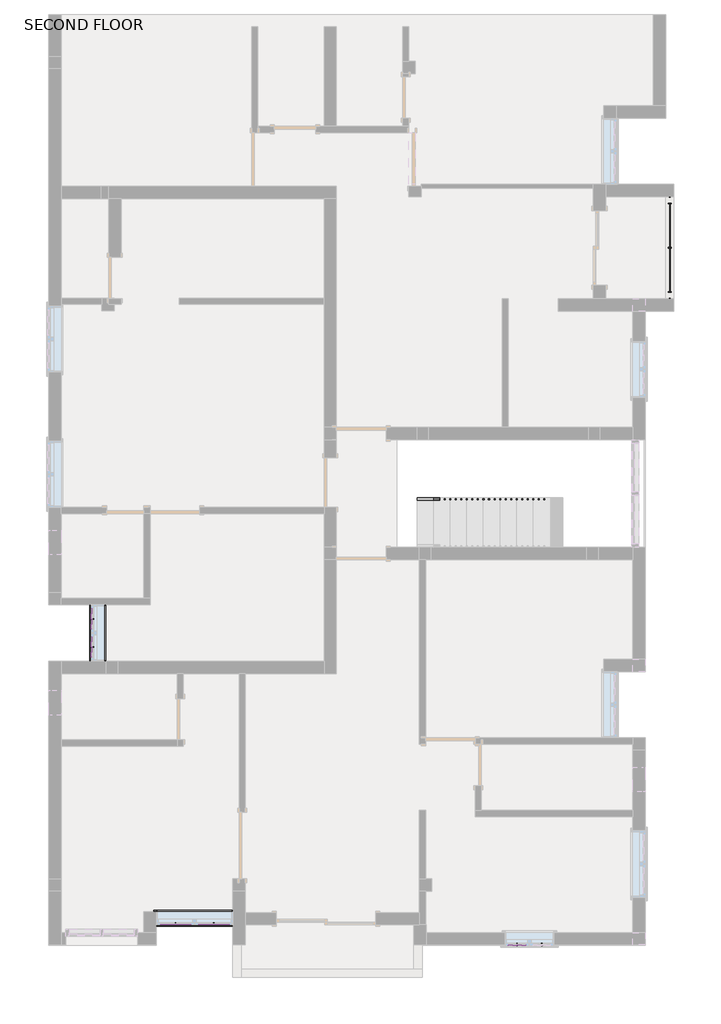
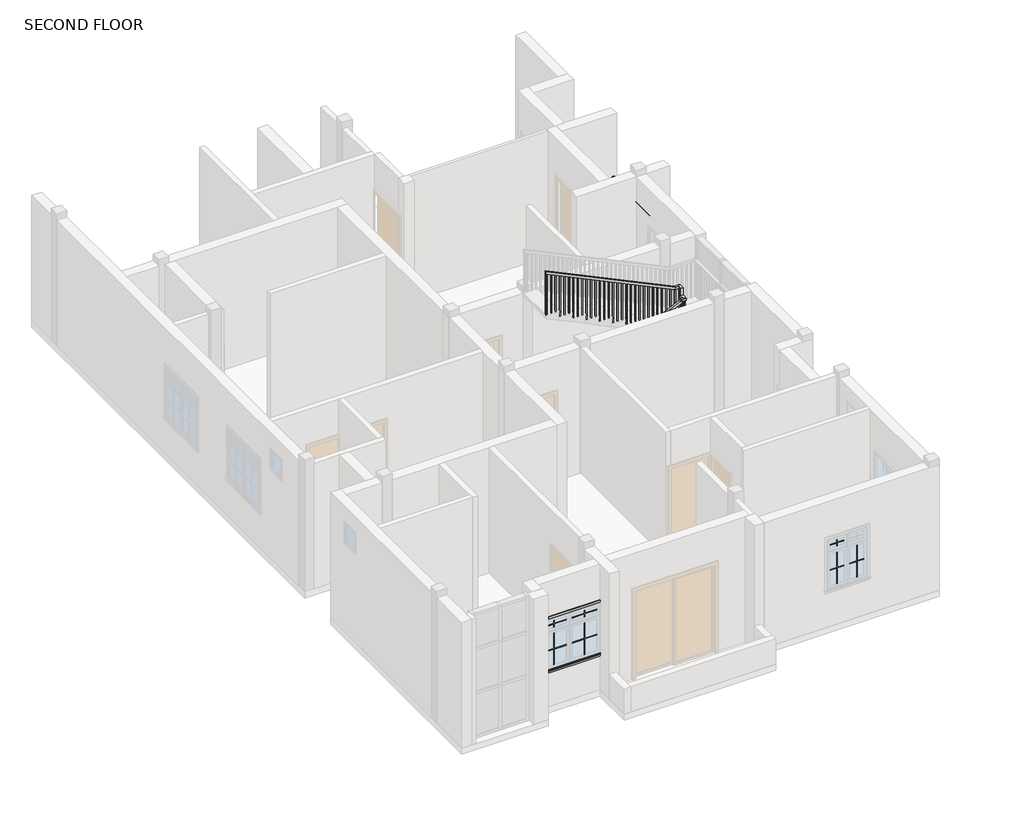
# One storey, part 5 of 6: 15 proxies, 2 railings.
"""IFC4 building model written with IfcOpenShell, lengths in millimetres."""

from ifc_helpers import new_model, si_unit, point, frame, origin, place, context, project, spatial, polyline, ellipse_curve, trimmed, outline, extrude, faceted_brep, transform, mapped, element, save
from ifc_brep_helpers import plane_surface, extruded_surface, advanced_brep
from components import muntin_pattern_2x2_muntin_pattern_2x2_a154cbfa, muntin_pattern_2x2_muntin_pattern_2x2_fbb866f2, muntin_pattern_2x2_muntin_pattern_2x2_1a5162a2, muntin_pattern_2x2_muntin_pattern_2x2_4af9dbf3, muntin_pattern_2x2_muntin_pattern_2x2_972acb6d, muntin_pattern_2x2_muntin_pattern_2x2_4879a4f3, muntin_pattern_2x2_muntin_pattern_2x2_d1c6e638, muntin_pattern_2x2_muntin_pattern_2x2_37b95fb2, muntin_pattern_2x2_muntin_pattern_2x2_604ffb00, trim_window_exterior_flat_with_sill_cb7cc766, trim_window_exterior_flat_with_sill_29d7a895, trim_window_interior_flat_picture_frame_9050e5f4, trim_window_interior_flat_picture_frame_56711e78

model = new_model("IFC4")

# Units and contexts
model_context = context("Model", 3, world=origin())
ifc_project = project(units=[si_unit("LENGTHUNIT", "METRE", prefix="MILLI")], contexts=[model_context])

# Site, building, storey
site = spatial("IfcSite", under=ifc_project)
building = spatial("IfcBuilding", under=site)
storey = spatial("IfcBuildingStorey", under=building, Name="SECOND FLOOR", Elevation=6400.8)

# Proxies
placement = place(None, origin())
muntin_pattern_2x2_muntin_pattern_2x2_shape = muntin_pattern_2x2_muntin_pattern_2x2_a154cbfa(model_context)
element("IfcBuildingElementProxy", 1, Name="Muntin Pattern_2x2 : Muntin Pattern_2x2", ObjectType="Muntin Pattern_2x2 : Muntin Pattern_2x2", at=placement, inside=storey, context=model_context, shape_type="MappedRepresentation", body=[
    mapped(muntin_pattern_2x2_muntin_pattern_2x2_shape, transform((-3731.5990981, -7428.8962413, 7385.05), x_axis=(-1.0, 0.0, 0.0), y_axis=(0.0, -1.0, 0.0), z_axis=(0.0, 0.0, 1.0))),
])
muntin_pattern_2x2_muntin_pattern_2x2_2_shape = muntin_pattern_2x2_muntin_pattern_2x2_fbb866f2(model_context)
element("IfcBuildingElementProxy", 2, Name="Muntin Pattern_2x2 : Muntin Pattern_2x2", ObjectType="Muntin Pattern_2x2 : Muntin Pattern_2x2", at=placement, inside=storey, context=model_context, shape_type="MappedRepresentation", body=[
    mapped(muntin_pattern_2x2_muntin_pattern_2x2_2_shape, transform((-4433.2740981, -7428.8962413, 7385.05), x_axis=(1.0, 0.0, 0.0), y_axis=(0.0, 1.0, 0.0), z_axis=(0.0, 0.0, 1.0))),
])
muntin_pattern_2x2_muntin_pattern_2x2_3_shape = muntin_pattern_2x2_muntin_pattern_2x2_1a5162a2(model_context)
element("IfcBuildingElementProxy", 3, Name="Muntin Pattern_2x2 : Muntin Pattern_2x2", ObjectType="Muntin Pattern_2x2 : Muntin Pattern_2x2", at=placement, inside=storey, context=model_context, shape_type="MappedRepresentation", body=[
    mapped(muntin_pattern_2x2_muntin_pattern_2x2_3_shape, transform((-4433.2740981, -7428.8962413, 8299.45), x_axis=(1.0, 0.0, 0.0), y_axis=(0.0, 1.0, 0.0), z_axis=(0.0, 0.0, 1.0))),
])
element("IfcBuildingElementProxy", 4, Name="Muntin Pattern_2x2 : Muntin Pattern_2x2", ObjectType="Muntin Pattern_2x2 : Muntin Pattern_2x2", at=placement, inside=storey, context=model_context, shape_type="MappedRepresentation", body=[
    mapped(muntin_pattern_2x2_muntin_pattern_2x2_3_shape, transform((-3731.5990981, -7428.8962413, 8299.45), x_axis=(1.0, 0.0, 0.0), y_axis=(0.0, 1.0, 0.0), z_axis=(0.0, 0.0, 1.0))),
])
muntin_pattern_2x2_muntin_pattern_2x2_4_shape = muntin_pattern_2x2_muntin_pattern_2x2_4af9dbf3(model_context)
element("IfcBuildingElementProxy", 5, Name="Muntin Pattern_2x2 : Muntin Pattern_2x2", ObjectType="Muntin Pattern_2x2 : Muntin Pattern_2x2", at=placement, inside=storey, context=model_context, shape_type="MappedRepresentation", body=[
    mapped(muntin_pattern_2x2_muntin_pattern_2x2_4_shape, transform((-5964.7636947, -2337.7837413, 7385.05), x_axis=(0.0, 1.0, 0.0), y_axis=(-1.0, 0.0, 0.0), z_axis=(0.0, 0.0, 1.0))),
])
muntin_pattern_2x2_muntin_pattern_2x2_5_shape = muntin_pattern_2x2_muntin_pattern_2x2_972acb6d(model_context)
element("IfcBuildingElementProxy", 6, Name="Muntin Pattern_2x2 : Muntin Pattern_2x2", ObjectType="Muntin Pattern_2x2 : Muntin Pattern_2x2", at=placement, inside=storey, context=model_context, shape_type="MappedRepresentation", body=[
    mapped(muntin_pattern_2x2_muntin_pattern_2x2_5_shape, transform((-5964.7636947, -1820.2587413, 7385.05), x_axis=(0.0, -1.0, 0.0), y_axis=(1.0, 0.0, 0.0), z_axis=(0.0, 0.0, 1.0))),
])
muntin_pattern_2x2_muntin_pattern_2x2_6_shape = muntin_pattern_2x2_muntin_pattern_2x2_4879a4f3(model_context)
element("IfcBuildingElementProxy", 7, Name="Muntin Pattern_2x2 : Muntin Pattern_2x2", ObjectType="Muntin Pattern_2x2 : Muntin Pattern_2x2", at=placement, inside=storey, context=model_context, shape_type="MappedRepresentation", body=[
    mapped(muntin_pattern_2x2_muntin_pattern_2x2_6_shape, transform((-5964.7636947, -1820.2587413, 8299.45), x_axis=(0.0, -1.0, 0.0), y_axis=(1.0, 0.0, 0.0), z_axis=(0.0, 0.0, 1.0))),
])
element("IfcBuildingElementProxy", 8, Name="Muntin Pattern_2x2 : Muntin Pattern_2x2", ObjectType="Muntin Pattern_2x2 : Muntin Pattern_2x2", at=placement, inside=storey, context=model_context, shape_type="MappedRepresentation", body=[
    mapped(muntin_pattern_2x2_muntin_pattern_2x2_6_shape, transform((-5964.7636947, -2337.7837413, 8299.45), x_axis=(0.0, -1.0, 0.0), y_axis=(1.0, 0.0, 0.0), z_axis=(0.0, 0.0, 1.0))),
])
muntin_pattern_2x2_muntin_pattern_2x2_7_shape = muntin_pattern_2x2_muntin_pattern_2x2_d1c6e638(model_context)
element("IfcBuildingElementProxy", 9, Name="Muntin Pattern_2x2 : Muntin Pattern_2x2", ObjectType="Muntin Pattern_2x2 : Muntin Pattern_2x2", at=placement, inside=storey, context=model_context, shape_type="MappedRepresentation", body=[
    mapped(muntin_pattern_2x2_muntin_pattern_2x2_7_shape, transform((2304.0759019, -7809.8962413, 7385.05), x_axis=(-1.0, 0.0, 0.0), y_axis=(0.0, -1.0, 0.0), z_axis=(0.0, 0.0, 1.0))),
])
muntin_pattern_2x2_muntin_pattern_2x2_8_shape = muntin_pattern_2x2_muntin_pattern_2x2_37b95fb2(model_context)
element("IfcBuildingElementProxy", 10, Name="Muntin Pattern_2x2 : Muntin Pattern_2x2", ObjectType="Muntin Pattern_2x2 : Muntin Pattern_2x2", at=placement, inside=storey, context=model_context, shape_type="MappedRepresentation", body=[
    mapped(muntin_pattern_2x2_muntin_pattern_2x2_8_shape, transform((1850.0509019, -7809.8962413, 7385.05), x_axis=(1.0, 0.0, 0.0), y_axis=(0.0, 1.0, 0.0), z_axis=(0.0, 0.0, 1.0))),
])
muntin_pattern_2x2_muntin_pattern_2x2_9_shape = muntin_pattern_2x2_muntin_pattern_2x2_604ffb00(model_context)
element("IfcBuildingElementProxy", 11, Name="Muntin Pattern_2x2 : Muntin Pattern_2x2", ObjectType="Muntin Pattern_2x2 : Muntin Pattern_2x2", at=placement, inside=storey, context=model_context, shape_type="MappedRepresentation", body=[
    mapped(muntin_pattern_2x2_muntin_pattern_2x2_9_shape, transform((1850.0509019, -7809.8962413, 8299.45), x_axis=(1.0, 0.0, 0.0), y_axis=(0.0, 1.0, 0.0), z_axis=(0.0, 0.0, 1.0))),
])
trim_window_exterior_flat_with_sill_shape = trim_window_exterior_flat_with_sill_cb7cc766(model_context)
element("IfcBuildingElementProxy", 12, Name="Trim-Window-Exterior-Flat : with Sill", ObjectType="Trim-Window-Exterior-Flat : with Sill", at=placement, inside=storey, context=model_context, shape_type="MappedRepresentation", body=[
    mapped(trim_window_exterior_flat_with_sill_shape, transform((-4082.4365981, -7438.4212413, 8534.4), x_axis=(1.0, 0.0, 0.0), y_axis=(0.0, 0.0, 1.0), z_axis=(0.0, -1.0, 0.0))),
])
trim_window_exterior_flat_with_sill_2_shape = trim_window_exterior_flat_with_sill_29d7a895(model_context)
element("IfcBuildingElementProxy", 13, Name="Trim-Window-Exterior-Flat : with Sill", ObjectType="Trim-Window-Exterior-Flat : with Sill", at=placement, inside=storey, context=model_context, shape_type="MappedRepresentation", body=[
    mapped(trim_window_exterior_flat_with_sill_2_shape, transform((-5974.2886947, -2079.0212413, 8534.4), x_axis=(0.0, -1.0, 0.0), y_axis=(0.0, 0.0, 1.0), z_axis=(-1.0, 0.0, 0.0))),
])
trim_window_interior_flat_picture_frame_shape = trim_window_interior_flat_picture_frame_9050e5f4(model_context)
element("IfcBuildingElementProxy", 14, Name="Trim-Window-Interior-Flat : Picture Frame", ObjectType="Trim-Window-Interior-Flat : Picture Frame", at=placement, inside=storey, context=model_context, shape_type="MappedRepresentation", body=[
    mapped(trim_window_interior_flat_picture_frame_shape, transform((-4082.4365981, -7209.8212413, 8534.4), x_axis=(-1.0, 0.0, 0.0), y_axis=(0.0, 0.0, 1.0), z_axis=(0.0, 1.0, 0.0))),
])
trim_window_interior_flat_picture_frame_2_shape = trim_window_interior_flat_picture_frame_56711e78(model_context)
element("IfcBuildingElementProxy", 15, Name="Trim-Window-Interior-Flat : Picture Frame", ObjectType="Trim-Window-Interior-Flat : Picture Frame", at=placement, inside=storey, context=model_context, shape_type="MappedRepresentation", body=[
    mapped(trim_window_interior_flat_picture_frame_2_shape, transform((-5745.6886947, -2079.0212413, 8534.4), x_axis=(0.0, 1.0, 0.0), y_axis=(0.0, 0.0, 1.0), z_axis=(1.0, 0.0, 0.0))),
])

# Railings
element("IfcRailing", 16, ObjectType="Glass Panel - Bottom Fill", at=placement, inside=storey, context=model_context, shape_type="SolidModel", body=[
    advanced_brep(
    [(4699.6134019, 5947.3787587, 7924.8), (4623.4134019, 5947.3787587, 7924.8), (4699.6134019, 4067.7787587, 7924.8), (4623.4134019, 4067.7787587, 7924.8)],
    [
        (0, 1, ellipse_curve(frame((4661.5134019, 5947.3787587, 7924.8), z_axis=(0.0, 1.0, 0.0), x_axis=(-1.0, 0.0, 0.0)), 38.1, 28.575)),
        (1, 0, ellipse_curve(frame((4661.5134019, 5947.3787587, 7924.8), z_axis=(0.0, 1.0, 0.0), x_axis=(-1.0, 0.0, 0.0)), 38.1, 28.575)),
        (2, 3, ellipse_curve(frame((4661.5134019, 4067.7787587, 7924.8), z_axis=(0.0, -1.0, 0.0), x_axis=(-1.0, 0.0, 0.0)), 38.1, 28.575)),
        (3, 2, ellipse_curve(frame((4661.5134019, 4067.7787587, 7924.8), z_axis=(0.0, -1.0, 0.0), x_axis=(-1.0, 0.0, 0.0)), 38.1, 28.575)),
        (0, 2),
        (3, 1),
    ],
    [
        plane_surface(frame((4661.5134019, 5947.3787587, 7924.8), z_axis=(0.0, 1.0, 0.0), x_axis=(0.0, 0.0, -1.0))),
        plane_surface(frame((4661.5134019, 4067.7787587, 7924.8), z_axis=(0.0, -1.0, 0.0), x_axis=(0.0, 0.0, -1.0))),
        extruded_surface(trimmed(ellipse_curve(frame((4661.5134019, 4067.7787587, 7924.8), z_axis=(0.0, 1.0, 0.0), x_axis=(-1.0, 0.0, 0.0)), 38.1, 28.575), [point((4699.6134019, 4067.7787587, 7924.8))], [point((4623.4134019, 4067.7787587, 7924.8))], True, "CARTESIAN"), (0.0, 1879.6, 0.0), 1879.6),
        extruded_surface(trimmed(ellipse_curve(frame((4661.5134019, 4067.7787587, 7924.8), z_axis=(0.0, 1.0, 0.0), x_axis=(-1.0, 0.0, 0.0)), 38.1, 28.575), [point((4623.4134019, 4067.7787587, 7924.8))], [point((4699.6134019, 4067.7787587, 7924.8))], True, "CARTESIAN"), (0.0, 1879.6, 0.0), 1879.6),
    ],
    [
        (0, [[1, 2]]),
        (1, [[3, 4]]),
        (2, [[-1, 5, -4, 6]]),
        (3, [[-2, -6, -3, -5]]),
    ],
),
    extrude(outline(polyline([(4648.8134019, 5947.3787587), (4674.2134019, 5947.3787587), (4674.2134019, 4067.7787587), (4648.8134019, 4067.7787587), (4648.8134019, 5947.3787587)])), frame((0.0, 0.0, 7810.5), z_axis=(0.0, 0.0, 1.0), x_axis=(1.0, 0.0, 0.0)), (0.0, 0.0, 1.0), 25.4),
    extrude(outline(polyline([(4648.8134019, 5947.3787587), (4674.2134019, 5947.3787587), (4674.2134019, 4067.7787587), (4648.8134019, 4067.7787587), (4648.8134019, 5947.3787587)])), frame((0.0, 0.0, 7708.9), z_axis=(0.0, 0.0, 1.0), x_axis=(1.0, 0.0, 0.0)), (0.0, 0.0, 1.0), 25.4),
    extrude(outline(polyline([(4636.1134019, 4201.1287587), (4686.9134019, 4201.1287587), (4686.9134019, 4188.4287587), (4636.1134019, 4188.4287587), (4636.1134019, 4201.1287587)])), frame((0.0, 0.0, 7010.4), z_axis=(0.0, 0.0, 1.0), x_axis=(1.0, 0.0, 0.0)), (0.0, 0.0, 1.0), 885.825),
    extrude(outline(polyline([(4668.0485589, 5007.5787587), (4668.0485589, 4194.7787587), (4661.6985589, 4194.7787587), (4661.6985589, 5007.5787587), (4668.0485589, 5007.5787587)])), frame((0.0, 0.0, 7112.0), z_axis=(0.0, 0.0, 1.0), x_axis=(1.0, 0.0, 0.0)), (0.0, 0.0, 1.0), 596.9),
    extrude(outline(polyline([(4636.1134019, 5013.9287587), (4686.9134019, 5013.9287587), (4686.9134019, 5001.2287587), (4636.1134019, 5001.2287587), (4636.1134019, 5013.9287587)])), frame((0.0, 0.0, 7010.4), z_axis=(0.0, 0.0, 1.0), x_axis=(1.0, 0.0, 0.0)), (0.0, 0.0, 1.0), 885.825),
    extrude(outline(polyline([(4668.0485589, 5820.3787587), (4668.0485589, 5007.5787587), (4661.6985589, 5007.5787587), (4661.6985589, 5820.3787587), (4668.0485589, 5820.3787587)])), frame((0.0, 0.0, 7112.0), z_axis=(0.0, 0.0, 1.0), x_axis=(1.0, 0.0, 0.0)), (0.0, 0.0, 1.0), 596.9),
    extrude(outline(polyline([(4636.1134019, 5826.7287587), (4686.9134019, 5826.7287587), (4686.9134019, 5814.0287587), (4636.1134019, 5814.0287587), (4636.1134019, 5826.7287587)])), frame((0.0, 0.0, 7010.4), z_axis=(0.0, 0.0, 1.0), x_axis=(1.0, 0.0, 0.0)), (0.0, 0.0, 1.0), 885.825),
    extrude(outline(polyline([(4651.9884019, 4080.4787587), (4671.0384019, 4080.4787587), (4671.0384019, 4061.4287587), (4651.9884019, 4061.4287587), (4651.9884019, 4080.4787587)])), frame((0.0, 0.0, 7010.4), z_axis=(0.0, 0.0, 1.0), x_axis=(1.0, 0.0, 0.0)), (0.0, 0.0, 1.0), 885.825),
    extrude(outline(polyline([(4651.9884019, 5953.7287587), (4671.0384019, 5953.7287587), (4671.0384019, 5934.6787587), (4651.9884019, 5934.6787587), (4651.9884019, 5953.7287587)])), frame((0.0, 0.0, 7010.4), z_axis=(0.0, 0.0, 1.0), x_axis=(1.0, 0.0, 0.0)), (0.0, 0.0, 1.0), 885.825),
])
element("IfcRailing", 17, ObjectType="Handrail - Rectangular", at=placement, inside=storey, context=model_context, shape_type="SolidModel", body=[
    faceted_brep([(13.3134019, 410.1787587, 7460.6727273), (13.3134019, 410.1787587, 7404.3834559), (13.3134019, 359.3787587, 7404.3834559), (13.3134019, 359.3787587, 7460.6727273), (2985.1134019, 410.1787587, 8879.0318182), (3035.9134019, 410.1787587, 8846.9880014), (3035.9134019, 359.3787587, 8846.9880014), (2985.1134019, 359.3787587, 8879.0318182), (2985.1134019, 410.1787587, 8915.4), (3035.9134019, 410.1787587, 8864.6), (3035.9134019, 359.3787587, 8864.6), (2985.1134019, 359.3787587, 8915.4), (3061.3134019, 410.1787587, 8915.4), (3061.3134019, 410.1787587, 8864.6), (3112.1134019, 359.3787587, 8864.6), (3112.1134019, 359.3787587, 8915.4), (3061.3134019, 486.3787587, 8915.4), (3061.3134019, 537.1787587, 8864.6), (3112.1134019, 537.1787587, 8864.6), (3112.1134019, 486.3787587, 8915.4), (3061.3134019, 486.3787587, 9097.2409091), (3061.3134019, 537.1787587, 9046.4409091), (3112.1134019, 537.1787587, 9046.4409091), (3112.1134019, 486.3787587, 9097.2409091), (3061.3134019, 562.5787587, 9097.2409091), (3061.3134019, 562.5787587, 9046.4409091), (3112.1134019, 613.3787587, 9046.4409091), (3112.1134019, 613.3787587, 9097.2409091), (2985.1134019, 562.5787587, 9097.2409091), (2973.6120715, 562.5787587, 9046.4409091), (2973.6120715, 613.3787587, 9046.4409091), (2985.1134019, 613.3787587, 9097.2409091), (13.3134019, 562.5787587, 10515.6), (13.3134019, 613.3787587, 10515.6), (13.3134019, 613.3787587, 10459.3107287), (13.3134019, 562.5787587, 10459.3107287)], [[[0, 1, 2, 3]], [[1, 0, 4, 5]], [[2, 1, 5, 6]], [[3, 2, 6, 7]], [[0, 3, 7, 4]], [[5, 4, 8, 9]], [[6, 5, 9, 10]], [[7, 6, 10, 11]], [[4, 7, 11, 8]], [[9, 8, 12, 13]], [[10, 9, 13, 14]], [[11, 10, 14, 15]], [[8, 11, 15, 12]], [[13, 12, 16, 17]], [[14, 13, 17, 18]], [[15, 14, 18, 19]], [[12, 15, 19, 16]], [[17, 16, 20, 21]], [[18, 17, 21, 22]], [[19, 18, 22, 23]], [[16, 19, 23, 20]], [[21, 20, 24, 25]], [[22, 21, 25, 26]], [[23, 22, 26, 27]], [[20, 23, 27, 24]], [[25, 24, 28, 29]], [[26, 25, 29, 30]], [[27, 26, 30, 31]], [[24, 27, 31, 28]], [[32, 33, 34, 35]], [[29, 28, 32, 35]], [[30, 29, 35, 34]], [[31, 30, 34, 33]], [[28, 31, 33, 32]]]),
    extrude(outline(polyline([(10451.7340241, 29.1884019), (9455.7272727, 29.1884019), (9455.7272727, 48.2384019), (10442.6419787, 48.2384019), (10451.7340241, 29.1884019)])), frame((0.0, 578.4537587, 0.0), z_axis=(0.0, 1.0, 0.0), x_axis=(0.0, 0.0, 1.0)), (0.0, 0.0, 1.0), 19.05),
    extrude(outline(polyline([(10403.243115, 130.7884019), (9455.7272727, 130.7884019), (9455.7272727, 149.8384019), (10394.1510696, 149.8384019), (10403.243115, 130.7884019)])), frame((0.0, 578.4537587, 0.0), z_axis=(0.0, 1.0, 0.0), x_axis=(0.0, 0.0, 1.0)), (0.0, 0.0, 1.0), 19.05),
    extrude(outline(polyline([(10354.7522059, 232.3884019), (9455.7272727, 232.3884019), (9455.7272727, 251.4384019), (10345.6601605, 251.4384019), (10354.7522059, 232.3884019)])), frame((0.0, 578.4537587, 0.0), z_axis=(0.0, 1.0, 0.0), x_axis=(0.0, 0.0, 1.0)), (0.0, 0.0, 1.0), 19.05),
    extrude(outline(polyline([(10306.2612969, 333.9884019), (9310.2545455, 333.9884019), (9310.2545455, 353.0384019), (10297.1692514, 353.0384019), (10306.2612969, 333.9884019)])), frame((0.0, 578.4537587, 0.0), z_axis=(0.0, 1.0, 0.0), x_axis=(0.0, 0.0, 1.0)), (0.0, 0.0, 1.0), 19.05),
    extrude(outline(polyline([(10257.7703878, 435.5884019), (9310.2545455, 435.5884019), (9310.2545455, 454.6384019), (10248.6783423, 454.6384019), (10257.7703878, 435.5884019)])), frame((0.0, 578.4537587, 0.0), z_axis=(0.0, 1.0, 0.0), x_axis=(0.0, 0.0, 1.0)), (0.0, 0.0, 1.0), 19.05),
    extrude(outline(polyline([(10209.2794787, 537.1884019), (9310.2545455, 537.1884019), (9310.2545455, 556.2384019), (10200.1874332, 556.2384019), (10209.2794787, 537.1884019)])), frame((0.0, 578.4537587, 0.0), z_axis=(0.0, 1.0, 0.0), x_axis=(0.0, 0.0, 1.0)), (0.0, 0.0, 1.0), 19.05),
    extrude(outline(polyline([(10160.7885696, 638.7884019), (9164.7818182, 638.7884019), (9164.7818182, 657.8384019), (10151.6965241, 657.8384019), (10160.7885696, 638.7884019)])), frame((0.0, 578.4537587, 0.0), z_axis=(0.0, 1.0, 0.0), x_axis=(0.0, 0.0, 1.0)), (0.0, 0.0, 1.0), 19.05),
    extrude(outline(polyline([(10112.2976605, 740.3884019), (9164.7818182, 740.3884019), (9164.7818182, 759.4384019), (10103.205615, 759.4384019), (10112.2976605, 740.3884019)])), frame((0.0, 578.4537587, 0.0), z_axis=(0.0, 1.0, 0.0), x_axis=(0.0, 0.0, 1.0)), (0.0, 0.0, 1.0), 19.05),
    extrude(outline(polyline([(10063.8067514, 841.9884019), (9164.7818182, 841.9884019), (9164.7818182, 861.0384019), (10054.7147059, 861.0384019), (10063.8067514, 841.9884019)])), frame((0.0, 578.4537587, 0.0), z_axis=(0.0, 1.0, 0.0), x_axis=(0.0, 0.0, 1.0)), (0.0, 0.0, 1.0), 19.05),
    extrude(outline(polyline([(10015.3158423, 943.5884019), (9019.3090909, 943.5884019), (9019.3090909, 962.6384019), (10006.2237969, 962.6384019), (10015.3158423, 943.5884019)])), frame((0.0, 578.4537587, 0.0), z_axis=(0.0, 1.0, 0.0), x_axis=(0.0, 0.0, 1.0)), (0.0, 0.0, 1.0), 19.05),
    extrude(outline(polyline([(9966.8249332, 1045.1884019), (9019.3090909, 1045.1884019), (9019.3090909, 1064.2384019), (9957.7328878, 1064.2384019), (9966.8249332, 1045.1884019)])), frame((0.0, 578.4537587, 0.0), z_axis=(0.0, 1.0, 0.0), x_axis=(0.0, 0.0, 1.0)), (0.0, 0.0, 1.0), 19.05),
    extrude(outline(polyline([(9918.3340241, 1146.7884019), (9019.3090909, 1146.7884019), (9019.3090909, 1165.8384019), (9909.2419787, 1165.8384019), (9918.3340241, 1146.7884019)])), frame((0.0, 578.4537587, 0.0), z_axis=(0.0, 1.0, 0.0), x_axis=(0.0, 0.0, 1.0)), (0.0, 0.0, 1.0), 19.05),
    extrude(outline(polyline([(9869.843115, 1248.3884019), (8873.8363636, 1248.3884019), (8873.8363636, 1267.4384019), (9860.7510696, 1267.4384019), (9869.843115, 1248.3884019)])), frame((0.0, 578.4537587, 0.0), z_axis=(0.0, 1.0, 0.0), x_axis=(0.0, 0.0, 1.0)), (0.0, 0.0, 1.0), 19.05),
    extrude(outline(polyline([(9821.3522059, 1349.9884019), (8873.8363636, 1349.9884019), (8873.8363636, 1369.0384019), (9812.2601605, 1369.0384019), (9821.3522059, 1349.9884019)])), frame((0.0, 578.4537587, 0.0), z_axis=(0.0, 1.0, 0.0), x_axis=(0.0, 0.0, 1.0)), (0.0, 0.0, 1.0), 19.05),
    extrude(outline(polyline([(9772.8612969, 1451.5884019), (8873.8363636, 1451.5884019), (8873.8363636, 1470.6384019), (9763.7692514, 1470.6384019), (9772.8612969, 1451.5884019)])), frame((0.0, 578.4537587, 0.0), z_axis=(0.0, 1.0, 0.0), x_axis=(0.0, 0.0, 1.0)), (0.0, 0.0, 1.0), 19.05),
    extrude(outline(polyline([(9724.3703878, 1553.1884019), (8728.3636364, 1553.1884019), (8728.3636364, 1572.2384019), (9715.2783423, 1572.2384019), (9724.3703878, 1553.1884019)])), frame((0.0, 578.4537587, 0.0), z_axis=(0.0, 1.0, 0.0), x_axis=(0.0, 0.0, 1.0)), (0.0, 0.0, 1.0), 19.05),
    extrude(outline(polyline([(9675.8794787, 1654.7884019), (8728.3636364, 1654.7884019), (8728.3636364, 1673.8384019), (9666.7874332, 1673.8384019), (9675.8794787, 1654.7884019)])), frame((0.0, 578.4537587, 0.0), z_axis=(0.0, 1.0, 0.0), x_axis=(0.0, 0.0, 1.0)), (0.0, 0.0, 1.0), 19.05),
    extrude(outline(polyline([(9627.3885696, 1756.3884019), (8728.3636364, 1756.3884019), (8728.3636364, 1775.4384019), (9618.2965241, 1775.4384019), (9627.3885696, 1756.3884019)])), frame((0.0, 578.4537587, 0.0), z_axis=(0.0, 1.0, 0.0), x_axis=(0.0, 0.0, 1.0)), (0.0, 0.0, 1.0), 19.05),
    extrude(outline(polyline([(9578.8976605, 1857.9884019), (8582.8909091, 1857.9884019), (8582.8909091, 1877.0384019), (9569.805615, 1877.0384019), (9578.8976605, 1857.9884019)])), frame((0.0, 578.4537587, 0.0), z_axis=(0.0, 1.0, 0.0), x_axis=(0.0, 0.0, 1.0)), (0.0, 0.0, 1.0), 19.05),
    extrude(outline(polyline([(9530.4067514, 1959.5884019), (8582.8909091, 1959.5884019), (8582.8909091, 1978.6384019), (9521.3147059, 1978.6384019), (9530.4067514, 1959.5884019)])), frame((0.0, 578.4537587, 0.0), z_axis=(0.0, 1.0, 0.0), x_axis=(0.0, 0.0, 1.0)), (0.0, 0.0, 1.0), 19.05),
    extrude(outline(polyline([(9481.9158423, 2061.1884019), (8582.8909091, 2061.1884019), (8582.8909091, 2080.2384019), (9472.8237969, 2080.2384019), (9481.9158423, 2061.1884019)])), frame((0.0, 578.4537587, 0.0), z_axis=(0.0, 1.0, 0.0), x_axis=(0.0, 0.0, 1.0)), (0.0, 0.0, 1.0), 19.05),
    extrude(outline(polyline([(9433.4249332, 2162.7884019), (8437.4181818, 2162.7884019), (8437.4181818, 2181.8384019), (9424.3328878, 2181.8384019), (9433.4249332, 2162.7884019)])), frame((0.0, 578.4537587, 0.0), z_axis=(0.0, 1.0, 0.0), x_axis=(0.0, 0.0, 1.0)), (0.0, 0.0, 1.0), 19.05),
    extrude(outline(polyline([(9384.9340241, 2264.3884019), (8437.4181818, 2264.3884019), (8437.4181818, 2283.4384019), (9375.8419787, 2283.4384019), (9384.9340241, 2264.3884019)])), frame((0.0, 578.4537587, 0.0), z_axis=(0.0, 1.0, 0.0), x_axis=(0.0, 0.0, 1.0)), (0.0, 0.0, 1.0), 19.05),
    extrude(outline(polyline([(9336.443115, 2365.9884019), (8437.4181818, 2365.9884019), (8437.4181818, 2385.0384019), (9327.3510696, 2385.0384019), (9336.443115, 2365.9884019)])), frame((0.0, 578.4537587, 0.0), z_axis=(0.0, 1.0, 0.0), x_axis=(0.0, 0.0, 1.0)), (0.0, 0.0, 1.0), 19.05),
    extrude(outline(polyline([(9287.9522059, 2467.5884019), (8291.9454545, 2467.5884019), (8291.9454545, 2486.6384019), (9278.8601605, 2486.6384019), (9287.9522059, 2467.5884019)])), frame((0.0, 578.4537587, 0.0), z_axis=(0.0, 1.0, 0.0), x_axis=(0.0, 0.0, 1.0)), (0.0, 0.0, 1.0), 19.05),
    extrude(outline(polyline([(9239.4612969, 2569.1884019), (8291.9454545, 2569.1884019), (8291.9454545, 2588.2384019), (9230.3692514, 2588.2384019), (9239.4612969, 2569.1884019)])), frame((0.0, 578.4537587, 0.0), z_axis=(0.0, 1.0, 0.0), x_axis=(0.0, 0.0, 1.0)), (0.0, 0.0, 1.0), 19.05),
    extrude(outline(polyline([(9190.9703878, 2670.7884019), (8291.9454545, 2670.7884019), (8291.9454545, 2689.8384019), (9181.8783423, 2689.8384019), (9190.9703878, 2670.7884019)])), frame((0.0, 578.4537587, 0.0), z_axis=(0.0, 1.0, 0.0), x_axis=(0.0, 0.0, 1.0)), (0.0, 0.0, 1.0), 19.05),
    extrude(outline(polyline([(9142.4794787, 2772.3884019), (8146.4727273, 2772.3884019), (8146.4727273, 2791.4384019), (9133.3874332, 2791.4384019), (9142.4794787, 2772.3884019)])), frame((0.0, 578.4537587, 0.0), z_axis=(0.0, 1.0, 0.0), x_axis=(0.0, 0.0, 1.0)), (0.0, 0.0, 1.0), 19.05),
    extrude(outline(polyline([(9093.9885696, 2873.9884019), (8146.4727273, 2873.9884019), (8146.4727273, 2893.0384019), (9084.8965241, 2893.0384019), (9093.9885696, 2873.9884019)])), frame((0.0, 578.4537587, 0.0), z_axis=(0.0, 1.0, 0.0), x_axis=(0.0, 0.0, 1.0)), (0.0, 0.0, 1.0), 19.05),
    extrude(outline(polyline([(9045.4976605, 2975.5884019), (8146.4727273, 2975.5884019), (8146.4727273, 2994.6384019), (9036.405615, 2994.6384019), (9045.4976605, 2975.5884019)])), frame((0.0, 578.4537587, 0.0), z_axis=(0.0, 1.0, 0.0), x_axis=(0.0, 0.0, 1.0)), (0.0, 0.0, 1.0), 19.05),
    extrude(outline(polyline([(3077.1884019, 476.8537587), (3077.1884019, 495.9037587), (3096.2384019, 495.9037587), (3096.2384019, 476.8537587), (3077.1884019, 476.8537587)])), frame((0.0, 0.0, 8001.0), z_axis=(0.0, 0.0, 1.0), x_axis=(1.0, 0.0, 0.0)), (0.0, 0.0, 1.0), 863.6),
    extrude(outline(polyline([(3051.7884019, 394.3037587), (3070.8384019, 394.3037587), (3070.8384019, 375.2537587), (3051.7884019, 375.2537587), (3051.7884019, 394.3037587)])), frame((0.0, 0.0, 8001.0), z_axis=(0.0, 0.0, 1.0), x_axis=(1.0, 0.0, 0.0)), (0.0, 0.0, 1.0), 863.6),
    extrude(outline(polyline([(8806.0737969, 2950.1884019), (7855.5272727, 2950.1884019), (7855.5272727, 2969.2384019), (8815.1658423, 2969.2384019), (8806.0737969, 2950.1884019)])), frame((0.0, 375.2537587, 0.0), z_axis=(0.0, 1.0, 0.0), x_axis=(0.0, 0.0, 1.0)), (0.0, 0.0, 1.0), 19.05),
    extrude(outline(polyline([(8757.5828878, 2848.5884019), (7855.5272727, 2848.5884019), (7855.5272727, 2867.6384019), (8766.6749332, 2867.6384019), (8757.5828878, 2848.5884019)])), frame((0.0, 375.2537587, 0.0), z_axis=(0.0, 1.0, 0.0), x_axis=(0.0, 0.0, 1.0)), (0.0, 0.0, 1.0), 19.05),
    extrude(outline(polyline([(8709.0919787, 2746.9884019), (7855.5272727, 2746.9884019), (7855.5272727, 2766.0384019), (8718.1840241, 2766.0384019), (8709.0919787, 2746.9884019)])), frame((0.0, 375.2537587, 0.0), z_axis=(0.0, 1.0, 0.0), x_axis=(0.0, 0.0, 1.0)), (0.0, 0.0, 1.0), 19.05),
    extrude(outline(polyline([(8660.6010696, 2645.3884019), (7710.0545455, 2645.3884019), (7710.0545455, 2664.4384019), (8669.693115, 2664.4384019), (8660.6010696, 2645.3884019)])), frame((0.0, 375.2537587, 0.0), z_axis=(0.0, 1.0, 0.0), x_axis=(0.0, 0.0, 1.0)), (0.0, 0.0, 1.0), 19.05),
    extrude(outline(polyline([(8612.1101605, 2543.7884019), (7710.0545455, 2543.7884019), (7710.0545455, 2562.8384019), (8621.2022059, 2562.8384019), (8612.1101605, 2543.7884019)])), frame((0.0, 375.2537587, 0.0), z_axis=(0.0, 1.0, 0.0), x_axis=(0.0, 0.0, 1.0)), (0.0, 0.0, 1.0), 19.05),
    extrude(outline(polyline([(8563.6192514, 2442.1884019), (7710.0545455, 2442.1884019), (7710.0545455, 2461.2384019), (8572.7112969, 2461.2384019), (8563.6192514, 2442.1884019)])), frame((0.0, 375.2537587, 0.0), z_axis=(0.0, 1.0, 0.0), x_axis=(0.0, 0.0, 1.0)), (0.0, 0.0, 1.0), 19.05),
    extrude(outline(polyline([(8515.1283423, 2340.5884019), (7564.5818182, 2340.5884019), (7564.5818182, 2359.6384019), (8524.2203878, 2359.6384019), (8515.1283423, 2340.5884019)])), frame((0.0, 375.2537587, 0.0), z_axis=(0.0, 1.0, 0.0), x_axis=(0.0, 0.0, 1.0)), (0.0, 0.0, 1.0), 19.05),
    extrude(outline(polyline([(8466.6374332, 2238.9884019), (7564.5818182, 2238.9884019), (7564.5818182, 2258.0384019), (8475.7294787, 2258.0384019), (8466.6374332, 2238.9884019)])), frame((0.0, 375.2537587, 0.0), z_axis=(0.0, 1.0, 0.0), x_axis=(0.0, 0.0, 1.0)), (0.0, 0.0, 1.0), 19.05),
    extrude(outline(polyline([(8418.1465241, 2137.3884019), (7564.5818182, 2137.3884019), (7564.5818182, 2156.4384019), (8427.2385696, 2156.4384019), (8418.1465241, 2137.3884019)])), frame((0.0, 375.2537587, 0.0), z_axis=(0.0, 1.0, 0.0), x_axis=(0.0, 0.0, 1.0)), (0.0, 0.0, 1.0), 19.05),
    extrude(outline(polyline([(8369.655615, 2035.7884019), (7419.1090909, 2035.7884019), (7419.1090909, 2054.8384019), (8378.7476605, 2054.8384019), (8369.655615, 2035.7884019)])), frame((0.0, 375.2537587, 0.0), z_axis=(0.0, 1.0, 0.0), x_axis=(0.0, 0.0, 1.0)), (0.0, 0.0, 1.0), 19.05),
    extrude(outline(polyline([(8321.1647059, 1934.1884019), (7419.1090909, 1934.1884019), (7419.1090909, 1953.2384019), (8330.2567514, 1953.2384019), (8321.1647059, 1934.1884019)])), frame((0.0, 375.2537587, 0.0), z_axis=(0.0, 1.0, 0.0), x_axis=(0.0, 0.0, 1.0)), (0.0, 0.0, 1.0), 19.05),
    extrude(outline(polyline([(8272.6737969, 1832.5884019), (7419.1090909, 1832.5884019), (7419.1090909, 1851.6384019), (8281.7658423, 1851.6384019), (8272.6737969, 1832.5884019)])), frame((0.0, 375.2537587, 0.0), z_axis=(0.0, 1.0, 0.0), x_axis=(0.0, 0.0, 1.0)), (0.0, 0.0, 1.0), 19.05),
    extrude(outline(polyline([(8224.1828878, 1730.9884019), (7273.6363636, 1730.9884019), (7273.6363636, 1750.0384019), (8233.2749332, 1750.0384019), (8224.1828878, 1730.9884019)])), frame((0.0, 375.2537587, 0.0), z_axis=(0.0, 1.0, 0.0), x_axis=(0.0, 0.0, 1.0)), (0.0, 0.0, 1.0), 19.05),
    extrude(outline(polyline([(8175.6919787, 1629.3884019), (7273.6363636, 1629.3884019), (7273.6363636, 1648.4384019), (8184.7840241, 1648.4384019), (8175.6919787, 1629.3884019)])), frame((0.0, 375.2537587, 0.0), z_axis=(0.0, 1.0, 0.0), x_axis=(0.0, 0.0, 1.0)), (0.0, 0.0, 1.0), 19.05),
    extrude(outline(polyline([(8127.2010696, 1527.7884019), (7273.6363636, 1527.7884019), (7273.6363636, 1546.8384019), (8136.293115, 1546.8384019), (8127.2010696, 1527.7884019)])), frame((0.0, 375.2537587, 0.0), z_axis=(0.0, 1.0, 0.0), x_axis=(0.0, 0.0, 1.0)), (0.0, 0.0, 1.0), 19.05),
    extrude(outline(polyline([(8078.7101605, 1426.1884019), (7128.1636364, 1426.1884019), (7128.1636364, 1445.2384019), (8087.8022059, 1445.2384019), (8078.7101605, 1426.1884019)])), frame((0.0, 375.2537587, 0.0), z_axis=(0.0, 1.0, 0.0), x_axis=(0.0, 0.0, 1.0)), (0.0, 0.0, 1.0), 19.05),
    extrude(outline(polyline([(8030.2192514, 1324.5884019), (7128.1636364, 1324.5884019), (7128.1636364, 1343.6384019), (8039.3112969, 1343.6384019), (8030.2192514, 1324.5884019)])), frame((0.0, 375.2537587, 0.0), z_axis=(0.0, 1.0, 0.0), x_axis=(0.0, 0.0, 1.0)), (0.0, 0.0, 1.0), 19.05),
    extrude(outline(polyline([(7981.7283423, 1222.9884019), (7128.1636364, 1222.9884019), (7128.1636364, 1242.0384019), (7990.8203878, 1242.0384019), (7981.7283423, 1222.9884019)])), frame((0.0, 375.2537587, 0.0), z_axis=(0.0, 1.0, 0.0), x_axis=(0.0, 0.0, 1.0)), (0.0, 0.0, 1.0), 19.05),
    extrude(outline(polyline([(7933.2374332, 1121.3884019), (6982.6909091, 1121.3884019), (6982.6909091, 1140.4384019), (7942.3294787, 1140.4384019), (7933.2374332, 1121.3884019)])), frame((0.0, 375.2537587, 0.0), z_axis=(0.0, 1.0, 0.0), x_axis=(0.0, 0.0, 1.0)), (0.0, 0.0, 1.0), 19.05),
    extrude(outline(polyline([(7884.7465241, 1019.7884019), (6982.6909091, 1019.7884019), (6982.6909091, 1038.8384019), (7893.8385696, 1038.8384019), (7884.7465241, 1019.7884019)])), frame((0.0, 375.2537587, 0.0), z_axis=(0.0, 1.0, 0.0), x_axis=(0.0, 0.0, 1.0)), (0.0, 0.0, 1.0), 19.05),
    extrude(outline(polyline([(7836.255615, 918.1884019), (6982.6909091, 918.1884019), (6982.6909091, 937.2384019), (7845.3476605, 937.2384019), (7836.255615, 918.1884019)])), frame((0.0, 375.2537587, 0.0), z_axis=(0.0, 1.0, 0.0), x_axis=(0.0, 0.0, 1.0)), (0.0, 0.0, 1.0), 19.05),
    extrude(outline(polyline([(7787.7647059, 816.5884019), (6837.2181818, 816.5884019), (6837.2181818, 835.6384019), (7796.8567514, 835.6384019), (7787.7647059, 816.5884019)])), frame((0.0, 375.2537587, 0.0), z_axis=(0.0, 1.0, 0.0), x_axis=(0.0, 0.0, 1.0)), (0.0, 0.0, 1.0), 19.05),
    extrude(outline(polyline([(7739.2737969, 714.9884019), (6837.2181818, 714.9884019), (6837.2181818, 734.0384019), (7748.3658423, 734.0384019), (7739.2737969, 714.9884019)])), frame((0.0, 375.2537587, 0.0), z_axis=(0.0, 1.0, 0.0), x_axis=(0.0, 0.0, 1.0)), (0.0, 0.0, 1.0), 19.05),
    extrude(outline(polyline([(7690.7828878, 613.3884019), (6837.2181818, 613.3884019), (6837.2181818, 632.4384019), (7699.8749332, 632.4384019), (7690.7828878, 613.3884019)])), frame((0.0, 375.2537587, 0.0), z_axis=(0.0, 1.0, 0.0), x_axis=(0.0, 0.0, 1.0)), (0.0, 0.0, 1.0), 19.05),
    extrude(outline(polyline([(7642.2919787, 511.7884019), (6691.7454545, 511.7884019), (6691.7454545, 530.8384019), (7651.3840241, 530.8384019), (7642.2919787, 511.7884019)])), frame((0.0, 375.2537587, 0.0), z_axis=(0.0, 1.0, 0.0), x_axis=(0.0, 0.0, 1.0)), (0.0, 0.0, 1.0), 19.05),
    extrude(outline(polyline([(7593.8010696, 410.1884019), (6691.7454545, 410.1884019), (6691.7454545, 429.2384019), (7602.893115, 429.2384019), (7593.8010696, 410.1884019)])), frame((0.0, 375.2537587, 0.0), z_axis=(0.0, 1.0, 0.0), x_axis=(0.0, 0.0, 1.0)), (0.0, 0.0, 1.0), 19.05),
    extrude(outline(polyline([(7545.3101605, 308.5884019), (6691.7454545, 308.5884019), (6691.7454545, 327.6384019), (7554.4022059, 327.6384019), (7545.3101605, 308.5884019)])), frame((0.0, 375.2537587, 0.0), z_axis=(0.0, 1.0, 0.0), x_axis=(0.0, 0.0, 1.0)), (0.0, 0.0, 1.0), 19.05),
    extrude(outline(polyline([(7496.8192514, 206.9884019), (6546.2727273, 206.9884019), (6546.2727273, 226.0384019), (7505.9112969, 226.0384019), (7496.8192514, 206.9884019)])), frame((0.0, 375.2537587, 0.0), z_axis=(0.0, 1.0, 0.0), x_axis=(0.0, 0.0, 1.0)), (0.0, 0.0, 1.0), 19.05),
    extrude(outline(polyline([(7448.3283423, 105.3884019), (6546.2727273, 105.3884019), (6546.2727273, 124.4384019), (7457.4203878, 124.4384019), (7448.3283423, 105.3884019)])), frame((0.0, 375.2537587, 0.0), z_axis=(0.0, 1.0, 0.0), x_axis=(0.0, 0.0, 1.0)), (0.0, 0.0, 1.0), 19.05),
    extrude(outline(polyline([(3077.1884019, 578.4537587), (3077.1884019, 597.5037587), (3096.2384019, 597.5037587), (3096.2384019, 578.4537587), (3077.1884019, 578.4537587)])), frame((0.0, 0.0, 8001.0), z_axis=(0.0, 0.0, 1.0), x_axis=(1.0, 0.0, 0.0)), (0.0, 0.0, 1.0), 1045.4409091),
    extrude(outline(polyline([(3077.1884019, 394.3037587), (3096.2384019, 394.3037587), (3096.2384019, 375.2537587), (3077.1884019, 375.2537587), (3077.1884019, 394.3037587)])), frame((0.0, 0.0, 8001.0), z_axis=(0.0, 0.0, 1.0), x_axis=(1.0, 0.0, 0.0)), (0.0, 0.0, 1.0), 863.6),
    extrude(outline(polyline([(10459.3107287, 13.3134019), (9455.7272727, 13.3134019), (9455.7272727, 32.3634019), (10450.2186832, 32.3634019), (10459.3107287, 13.3134019)])), frame((0.0, 578.4537587, 0.0), z_axis=(0.0, 1.0, 0.0), x_axis=(0.0, 0.0, 1.0)), (0.0, 0.0, 1.0), 19.05),
    extrude(outline(polyline([(7404.3834559, 13.3134019), (6546.2727273, 13.3134019), (6546.2727273, 32.3634019), (7413.4755014, 32.3634019), (7404.3834559, 13.3134019)])), frame((0.0, 375.2537587, 0.0), z_axis=(0.0, 1.0, 0.0), x_axis=(0.0, 0.0, 1.0)), (0.0, 0.0, 1.0), 19.05),
])

save(model, "model.ifc")

# Revit data of these elements
# Type "Muntin Pattern_2x2 : Muntin Pattern_2x2"
#   Width [instance default] = 4' - 0"
#   Thickness = 0' - 0 1/2"
#   Height [instance default] = 4' - 0"
#   Distance = 0' - 0 3/4"
#   Interior Material [instance default] = none
#   Exterior Material [instance default] = none
#   Default Elevation = 0
# Type "Trim-Window-Exterior-Flat : with Sill"
#   Trim Width = 0' - 2 1/4"
#   Trim Thickness_Picture Frame = 0' - 1 1/4"
#   Trim Thickness_with Sill = 0' - 0 3/4"
#   Sill Thickness = 0' - 1 1/4"
#   Opening Width [instance default] = 2' - 0"
#   Opening Height [instance default] = 3' - 0"
#   Default Elevation = 4' - 0"
#   Sill = yes
#   Picture Frame = no
#   Trim Material [instance default] = none
# Type "Trim-Window-Interior-Flat : Picture Frame"
#   Trim Thickness_Picture Frame = 0' - 1 1/4"
#   Trim Width = 0' - 2 1/4"
#   Trim Thickness_with Sill = 0' - 0 3/4"
#   Sill Thickness = 0' - 1 1/4"
#   Opening Width [instance default] = 2' - 0"
#   Opening Height [instance default] = 3' - 0"
#   Default Elevation = 4' - 0"
#   Sill = no
#   Picture Frame = yes
#   Trim Material [instance default] = none
# Type "Glass Panel - Bottom Fill"
#   Assembly Code = "C2010400"
#   built-in parameter 1008612 = 0.0416667 (stored number, unit not read)
#   built-in parameter 1008611 = 0.0416667 (stored number, unit not read)
#   built-in parameter 1008609 = 0.333333 (stored number, unit not read)
#   built-in parameter 1008604 = 0.166667 (stored number, unit not read)
#   built-in parameter 1008603 = 0.166667 (stored number, unit not read)
#   Railing Height = 3' - 0"
#   built-in parameter 1008630 = 2
#   built-in parameter 1008610 = 2
#   built-in parameter 1008618 = Baluster - Square : 3/4"
# Type "Handrail - Rectangular"
#   Assembly Code = "C2010400"
#   built-in parameter 1008612 = 0.0416667 (stored number, unit not read)
#   built-in parameter 1008611 = 0.0416667 (stored number, unit not read)
#   built-in parameter 1008609 = 0.333333 (stored number, unit not read)
#   built-in parameter 1008604 = 0.166667 (stored number, unit not read)
#   built-in parameter 1008603 = 0.166667 (stored number, unit not read)
#   Railing Height = 3' - 0"
#   built-in parameter 1008630 = 2
#   built-in parameter 1008610 = 2
#   built-in parameter 1008618 = Baluster - Square : 3/4"
# Elements 1, 2 (IfcBuildingElementProxy, "Muntin Pattern_2x2 : Muntin Pattern_2x2")
#   Width = 1' - 10 3/8"
#   Height = 2' - 6 1/2"
#   Interior Material = Wood - Stained
#   Exterior Material = Clad - White
#   Phase Created = New Construction
#   Materials on its faces: "Clad - White", "Wood - Stained"
# Elements 3, 4 (IfcBuildingElementProxy, "Muntin Pattern_2x2 : Muntin Pattern_2x2")
#   Width = 1' - 10 3/8"
#   Height = 0' - 6 1/2"
#   Interior Material = Wood - Stained
#   Exterior Material = Clad - White
#   Phase Created = New Construction
#   Materials on its faces: "Clad - White", "Wood - Stained"
# Elements 5, 6 (IfcBuildingElementProxy, "Muntin Pattern_2x2 : Muntin Pattern_2x2")
#   Width = 1' - 3 1/8"
#   Height = 2' - 6 1/2"
#   Interior Material = Wood - Stained
#   Exterior Material = Clad - White
#   Phase Created = New Construction
#   Materials on its faces: "Clad - White", "Wood - Stained"
# Elements 7, 8 (IfcBuildingElementProxy, "Muntin Pattern_2x2 : Muntin Pattern_2x2")
#   Width = 1' - 3 1/8"
#   Height = 0' - 6 1/2"
#   Interior Material = Wood - Stained
#   Exterior Material = Clad - White
#   Phase Created = New Construction
#   Materials on its faces: "Clad - White", "Wood - Stained"
# Elements 9, 10 (IfcBuildingElementProxy, "Muntin Pattern_2x2 : Muntin Pattern_2x2")
#   Width = 1' - 0 5/8"
#   Height = 2' - 6 1/2"
#   Interior Material = Wood - Stained
#   Exterior Material = Clad - White
#   Phase Created = New Construction
#   Materials on its faces: "Clad - White", "Wood - Stained"
# Element 11 (IfcBuildingElementProxy, "Muntin Pattern_2x2 : Muntin Pattern_2x2")
#   Width = 1' - 0 5/8"
#   Height = 0' - 6 1/2"
#   Interior Material = Wood - Stained
#   Exterior Material = Clad - White
#   Phase Created = New Construction
#   Materials on its faces: "Clad - White", "Wood - Stained"
# Element 12 (IfcBuildingElementProxy, "Trim-Window-Exterior-Flat : with Sill")
#   Opening Width = 4' - 7 1/2"
#   Opening Height = 4' - 0"
#   Trim Material = Clad - White
#   Phase Created = New Construction
#   Materials on its faces: "Clad - White"
# Element 13 (IfcBuildingElementProxy, "Trim-Window-Exterior-Flat : with Sill")
#   Opening Width = 3' - 5"
#   Opening Height = 4' - 0"
#   Trim Material = Clad - White
#   Phase Created = New Construction
#   Materials on its faces: "Clad - White"
# Element 14 (IfcBuildingElementProxy, "Trim-Window-Interior-Flat : Picture Frame")
#   Opening Width = 4' - 7 1/2"
#   Opening Height = 4' - 0"
#   Trim Material = Wood - Stained
#   Phase Created = New Construction
#   Materials on its faces: "Wood - Stained"
# Element 15 (IfcBuildingElementProxy, "Trim-Window-Interior-Flat : Picture Frame")
#   Opening Width = 3' - 5"
#   Opening Height = 4' - 0"
#   Trim Material = Wood - Stained
#   Phase Created = New Construction
#   Materials on its faces: "Wood - Stained"
# Element 16 (IfcRailing, "Glass Panel - Bottom Fill")
#   built-in parameter 1008621 = 2 (stored number, unit not read)
#   Phase Created = New Construction
#   Materials on its faces: "Glass"
# Element 17 (IfcRailing, "Handrail - Rectangular")
#   Phase Created = New Construction
# Materials
#   "Clad - White": class "Wood", colour RGB 242 242 238, transparency 0, Cost = 0
#   "Wood - Stained": class "Wood", colour RGB 224 178 126, transparency 0, Cost = 0
#   "Glass": class "Glass", colour RGB 0 128 192, transparency 0.75, Description = "Soda Lime Glass", Cost = 0
